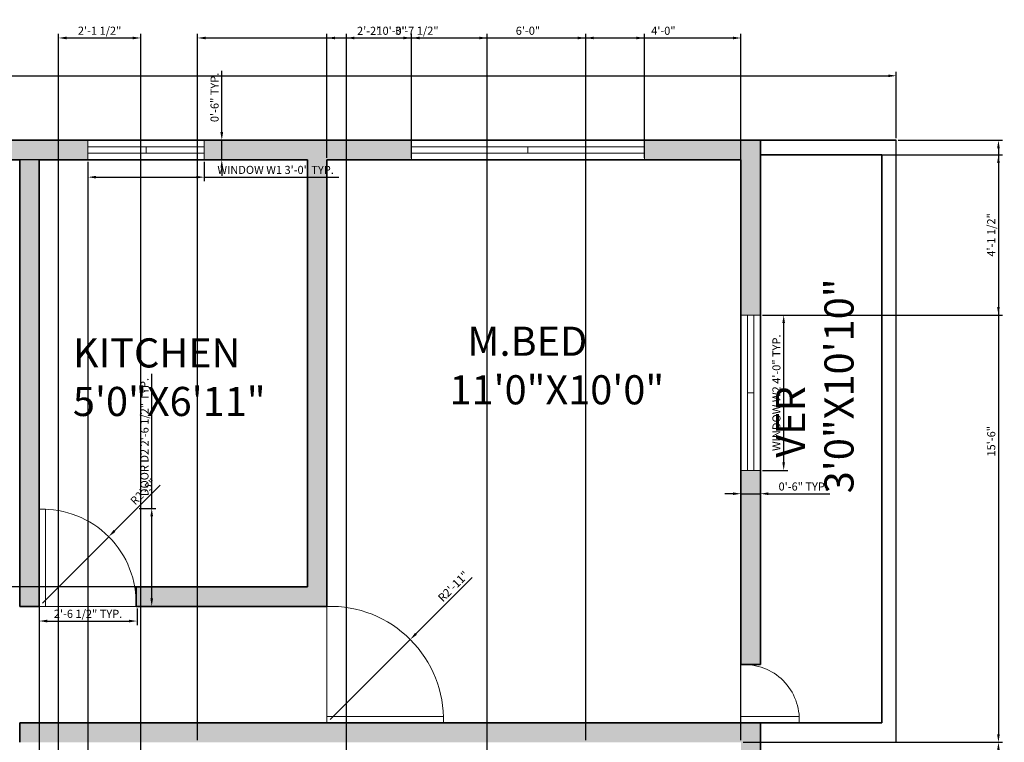
# Model space of a CAD drawing. Units: inches. Extents: x 5145 to 5807, y 9597 to 10060.
# Tile 3 of 3: x 5502 to 5807, y 9836 to 10060. Entities that reach past the tile are written whole.
import ezdxf

# ---------------------------------------------------------------- set-up
doc = ezdxf.new("R2010")
doc.units = ezdxf.units.IN
for name, color, linetype, lineweight in [('A-ANNO-DIMS', 7, 'Continuous', 18), ('A-AREA-IDEN', 7, 'Continuous', 18), ('A-GLAZ', 140, 'Continuous', 18), ('A-WALL', 7, 'Continuous', 35)]:
    doc.layers.add(name, color=color, linetype=linetype, lineweight=lineweight)
for name, color, linetype, lineweight, true_color in [('A-DOOR', 2, 'Continuous', 18, 0xf1eb1f), ('A-WALL-PATT', 159, 'Continuous', 13, 0x22346e), ('A-WALL-PRPT', 61, 'Continuous', 25, 0xedee99)]:
    doc.layers.add(name, color=color, linetype=linetype, lineweight=lineweight, true_color=true_color)
doc.styles.get("Standard").update_dxf_attribs({"font": 'arial.ttf'})
doc.dimstyles.new('ISO-25', dxfattribs={"dimtxt": 2.5, "dimasz": 2.5, "dimexe": 1.25, "dimexo": 0.625, "dimtad": 1, "dimlunit": 3, "dimtxsty": 'Standard', "dimcen": 2.5, "dimadec": 0, "dimazin": 0, "dimtfac": 1, "dimtmove": 0, "dimatfit": 3, "dimfxl": 1, "dimarcsym": 0})

# ---------------------------------------------------------------- blocks, each defined once
blk = doc.blocks.new('*D1')
at = {"layer": 'A-ANNO-DIMS', "color": 0, "lineweight": -2, "transparency": 16777216}
for p, q in [((5182.12, 10022.89), (5182.12, 10043.44)), ((5773.12, 10022.89), (5773.12, 10043.44)), ((5184.62, 10042.19), (5770.62, 10042.19))]:
    blk.add_line(p, q, dxfattribs=at)
at = {"layer": 'A-ANNO-DIMS', "color": 0, "transparency": 16777216}
for points in [[(5184.62, 10042.6), (5184.62, 10041.77), (5182.12, 10042.19)], [(5770.62, 10042.6), (5770.62, 10041.77), (5773.12, 10042.19)]]:
    blk.add_solid(points, dxfattribs=at)
at = {"layer": 'Defpoints', "color": 0, "transparency": 16777216}
for p in [(5773.12, 10042.19), (5182.12, 10022.27), (5773.12, 10022.27)]:
    blk.add_point(p, dxfattribs=at)
at = {"layer": 'A-ANNO-DIMS', "color": 0, "transparency": 16777216, "insert": (5477.62, 10047.41), "char_height": 9, "attachment_point": 5}
blk.add_mtext('49\'-3"', dxfattribs=at)
blk = doc.blocks.new('WIN-36IN')
for p, q in [((0, 6), (0, 0)), ((0, 6), (36, 6)), ((0, 4), (36, 4)), ((18, 2), (18, 4)), ((36, 0), (36, 6)), ((0, 2), (36, 2)), ((36, 0), (0, 0))]:
    blk.add_line(p, q)
blk = doc.blocks.new('WIN-48IN')
for p, q in [((6, 48), (0, 48)), ((0, 48), (0, 0)), ((2, 0), (2, 48)), ((4, 0), (4, 48)), ((6, 0), (6, 48)), ((4, 24), (2, 24)), ((0, 0), (6, 0))]:
    blk.add_line(p, q)
blk = doc.blocks.new('DOOR-SWING-18IN')
for p, q in [((0.03, 18.03), (18.03, 18.03)), ((16.03, 0.03), (16.03, 18.03)), ((16.03, 18.03), (18.03, 18.03)), ((18.03, 18.03), (18.03, 0.03)), ((18.03, 0.03), (16.03, 0.03))]:
    blk.add_line(p, q)
blk.add_arc((17.03, 17.03), 17.03, 176.6335, 273.3665)
blk = doc.blocks.new('DOOR-SWING-30IN')
for p, q in [((0, 0), (0, 30)), ((0, 30), (2, 30)), ((2, 30), (2, 0)), ((2, 0), (0, 0)), ((0, 0), (30, 0))]:
    blk.add_line(p, q)
blk.add_arc((1, 1), 29.02, 358.0251, 91.9749)
blk = doc.blocks.new('*D9')
at = {"layer": 'A-ANNO-DIMS', "color": 0, "lineweight": -2, "transparency": 16777216}
for p, q in [((5523.2, 10015.64), (5523.2, 10009.62)), ((5559.2, 10015.64), (5559.2, 10009.62)), ((5525.7, 10010.87), (5556.7, 10010.87)), ((5559.2, 10010.87), (5600.79, 10010.87))]:
    blk.add_line(p, q, dxfattribs=at)
at = {"layer": 'A-ANNO-DIMS', "color": 0, "transparency": 16777216}
for points in [[(5525.7, 10011.28), (5525.7, 10010.45), (5523.2, 10010.87)], [(5556.7, 10011.28), (5556.7, 10010.45), (5559.2, 10010.87)]]:
    blk.add_solid(points, dxfattribs=at)
at = {"layer": 'Defpoints', "color": 0, "transparency": 16777216}
for p in [(5523.2, 10016.27), (5559.2, 10016.27), (5559.2, 10010.87)]:
    blk.add_point(p, dxfattribs=at)
at = {"layer": 'A-ANNO-DIMS', "color": 0, "transparency": 16777216, "insert": (5581.24, 10012.79), "char_height": 2.5, "attachment_point": 5}
blk.add_mtext('WINDOW W1 3\'-0" TYP.', dxfattribs=at)
blk = doc.blocks.new('*D10')
at = {"layer": 'A-ANNO-DIMS', "color": 0, "lineweight": -2, "transparency": 16777216}
for p, q in [((5564.6, 10024.77), (5564.6, 10043.76)), ((5559.82, 10022.27), (5565.85, 10022.27)), ((5564.6, 10016.27), (5564.6, 10022.27)), ((5559.82, 10016.27), (5565.85, 10016.27)), ((5564.6, 10013.77), (5564.6, 10011.27))]:
    blk.add_line(p, q, dxfattribs=at)
at = {"layer": 'A-ANNO-DIMS', "color": 0, "transparency": 16777216}
for points in [[(5564.18, 10024.77), (5565.01, 10024.77), (5564.6, 10022.27)], [(5564.18, 10013.77), (5565.01, 10013.77), (5564.6, 10016.27)]]:
    blk.add_solid(points, dxfattribs=at)
at = {"layer": 'Defpoints', "color": 0, "transparency": 16777216}
for p in [(5559.2, 10022.27), (5564.6, 10022.27), (5559.2, 10016.27)]:
    blk.add_point(p, dxfattribs=at)
at = {"layer": 'A-ANNO-DIMS', "color": 0, "transparency": 16777216, "insert": (5562.69, 10035.51), "char_height": 2.5, "attachment_point": 5, "rotation": 90}
blk.add_mtext('0\'-6" TYP.', dxfattribs=at)
blk = doc.blocks.new('*D11')
at = {"layer": 'A-ANNO-DIMS', "color": 0, "lineweight": -2, "transparency": 16777216}
for p, q in [((5731.74, 9968.27), (5739.57, 9968.27)), ((5738.32, 9922.77), (5738.32, 9965.77)), ((5731.74, 9920.27), (5739.57, 9920.27))]:
    blk.add_line(p, q, dxfattribs=at)
at = {"layer": 'A-ANNO-DIMS', "color": 0, "transparency": 16777216}
for points in [[(5737.9, 9965.77), (5738.73, 9965.77), (5738.32, 9968.27)], [(5737.9, 9922.77), (5738.73, 9922.77), (5738.32, 9920.27)]]:
    blk.add_solid(points, dxfattribs=at)
at = {"layer": 'Defpoints', "color": 0, "transparency": 16777216}
for p in [(5731.12, 9968.27), (5738.32, 9968.27), (5731.12, 9920.27)]:
    blk.add_point(p, dxfattribs=at)
at = {"layer": 'A-ANNO-DIMS', "color": 0, "transparency": 16777216, "insert": (5736.4, 9944.27), "char_height": 2.5, "attachment_point": 5, "rotation": 90}
blk.add_mtext('WINDOW W2 4\'-0" TYP.', dxfattribs=at)
blk = doc.blocks.new('*D12')
at = {"layer": 'A-ANNO-DIMS', "color": 0, "lineweight": -2, "transparency": 16777216}
for p, q in [((5725.12, 9919.64), (5725.12, 9911.82)), ((5731.12, 9919.64), (5731.12, 9911.82)), ((5722.62, 9913.07), (5720.12, 9913.07)), ((5725.12, 9913.07), (5731.12, 9913.07)), ((5733.62, 9913.07), (5752.61, 9913.07))]:
    blk.add_line(p, q, dxfattribs=at)
at = {"layer": 'A-ANNO-DIMS', "color": 0, "transparency": 16777216}
for points in [[(5722.62, 9913.48), (5722.62, 9912.65), (5725.12, 9913.07)], [(5733.62, 9913.48), (5733.62, 9912.65), (5731.12, 9913.07)]]:
    blk.add_solid(points, dxfattribs=at)
at = {"layer": 'Defpoints', "color": 0, "transparency": 16777216}
for p in [(5725.12, 9920.27), (5731.12, 9920.27), (5731.12, 9913.07)]:
    blk.add_point(p, dxfattribs=at)
at = {"layer": 'A-ANNO-DIMS', "color": 0, "transparency": 16777216, "insert": (5744.36, 9914.97), "char_height": 2.5, "attachment_point": 5}
blk.add_mtext('0\'-6" TYP.', dxfattribs=at)
blk = doc.blocks.new('*D17')
at = {"layer": 'A-ANNO-DIMS', "color": 0, "lineweight": -2, "transparency": 16777216}
for p, q in [((5542.94, 9908.54), (5542.94, 9950.12)), ((5539.02, 9908.54), (5544.19, 9908.54)), ((5542.94, 9880.77), (5542.94, 9906.04)), ((5539.02, 9878.27), (5544.19, 9878.27))]:
    blk.add_line(p, q, dxfattribs=at)
at = {"layer": 'A-ANNO-DIMS', "color": 0, "transparency": 16777216}
for points in [[(5542.52, 9906.04), (5543.35, 9906.04), (5542.94, 9908.54)], [(5542.52, 9880.77), (5543.35, 9880.77), (5542.94, 9878.27)]]:
    blk.add_solid(points, dxfattribs=at)
at = {"layer": 'Defpoints', "color": 0, "transparency": 16777216}
for p in [(5538.39, 9908.54), (5542.94, 9908.54), (5538.39, 9878.27)]:
    blk.add_point(p, dxfattribs=at)
at = {"layer": 'A-ANNO-DIMS', "color": 0, "transparency": 16777216, "insert": (5541.02, 9930.58), "char_height": 2.5, "attachment_point": 5, "rotation": 90}
blk.add_mtext('DOOR D2 2\'-6 1/2" TYP.', dxfattribs=at)
blk = doc.blocks.new('*D18')
at = {"layer": 'A-ANNO-DIMS', "color": 0, "lineweight": -2, "transparency": 16777216}
for p, q in [((5508.12, 9877.64), (5508.12, 9872.48)), ((5538.39, 9877.64), (5538.39, 9872.48)), ((5510.62, 9873.73), (5535.89, 9873.73))]:
    blk.add_line(p, q, dxfattribs=at)
at = {"layer": 'A-ANNO-DIMS', "color": 0, "transparency": 16777216}
for points in [[(5510.62, 9874.14), (5510.62, 9873.31), (5508.12, 9873.73)], [(5535.89, 9874.14), (5535.89, 9873.31), (5538.39, 9873.73)]]:
    blk.add_solid(points, dxfattribs=at)
at = {"layer": 'Defpoints', "color": 0, "transparency": 16777216}
for p in [(5508.12, 9878.27), (5538.39, 9878.27), (5538.39, 9873.73)]:
    blk.add_point(p, dxfattribs=at)
at = {"layer": 'A-ANNO-DIMS', "color": 0, "transparency": 16777216, "insert": (5523.25, 9875.64), "char_height": 2.5, "attachment_point": 5}
blk.add_mtext('2\'-6 1/2" TYP.', dxfattribs=at)
blk = doc.blocks.new('*D27')
at = {"layer": 'A-ANNO-DIMS', "color": 0, "lineweight": -2, "transparency": 16777216}
for p, q in [((5773.74, 10022.27), (5805.97, 10022.27)), ((5804.72, 10019.77), (5804.72, 9838.77)), ((5773.74, 9836.27), (5805.97, 9836.27))]:
    blk.add_line(p, q, dxfattribs=at)
at = {"layer": 'A-ANNO-DIMS', "color": 0, "transparency": 16777216}
for points in [[(5804.3, 10019.77), (5805.13, 10019.77), (5804.72, 10022.27)], [(5804.3, 9838.77), (5805.13, 9838.77), (5804.72, 9836.27)]]:
    blk.add_solid(points, dxfattribs=at)
at = {"layer": 'Defpoints', "color": 0, "transparency": 16777216}
for p in [(5773.12, 10022.27), (5773.12, 9836.27), (5804.72, 9836.27)]:
    blk.add_point(p, dxfattribs=at)
at = {"layer": 'A-ANNO-DIMS', "color": 0, "transparency": 16777216, "insert": (5802.81, 9929.27), "char_height": 2.5, "attachment_point": 5, "rotation": 90}
blk.add_mtext('15\'-6"', dxfattribs=at)
blk = doc.blocks.new('*D29')
at = {"layer": 'A-ANNO-DIMS', "color": 0, "lineweight": -2, "transparency": 16777216}
for p, q in [((5590.49, 10016.27), (5149.27, 10016.27)), ((5150.52, 10013.77), (5150.52, 9886.77)), ((5590.49, 9884.27), (5149.27, 9884.27))]:
    blk.add_line(p, q, dxfattribs=at)
at = {"layer": 'A-ANNO-DIMS', "color": 0, "transparency": 16777216}
for points in [[(5150.1, 10013.77), (5150.93, 10013.77), (5150.52, 10016.27)], [(5150.1, 9886.77), (5150.93, 9886.77), (5150.52, 9884.27)]]:
    blk.add_solid(points, dxfattribs=at)
at = {"layer": 'Defpoints', "color": 0, "transparency": 16777216}
for p in [(5591.12, 10016.27), (5150.52, 9884.27), (5591.12, 9884.27)]:
    blk.add_point(p, dxfattribs=at)
at = {"layer": 'A-ANNO-DIMS', "color": 0, "transparency": 16777216, "insert": (5148.61, 9950.27), "char_height": 2.5, "attachment_point": 5, "rotation": 90}
blk.add_mtext('11\'-0"', dxfattribs=at)
blk = doc.blocks.new('*D31')
at = {"layer": 'A-ANNO-DIMS', "color": 0, "lineweight": -2, "transparency": 16777216}
for p, q in [((5557.12, 9836.89), (5557.12, 10055.12)), ((5677.12, 9836.89), (5677.12, 10055.12)), ((5559.62, 10053.87), (5674.62, 10053.87))]:
    blk.add_line(p, q, dxfattribs=at)
at = {"layer": 'A-ANNO-DIMS', "color": 0, "transparency": 16777216}
for points in [[(5559.62, 10054.28), (5559.62, 10053.45), (5557.12, 10053.87)], [(5674.62, 10054.28), (5674.62, 10053.45), (5677.12, 10053.87)]]:
    blk.add_solid(points, dxfattribs=at)
at = {"layer": 'Defpoints', "color": 0, "transparency": 16777216}
for p in [(5677.12, 10053.87), (5557.12, 9836.27), (5677.12, 9836.27)]:
    blk.add_point(p, dxfattribs=at)
at = {"layer": 'A-ANNO-DIMS', "color": 0, "transparency": 16777216, "insert": (5617.12, 10055.77), "char_height": 2.5, "attachment_point": 5}
blk.add_mtext('10\'-0"', dxfattribs=at)
blk = doc.blocks.new('*D32')
at = {"layer": 'A-ANNO-DIMS', "color": 0, "lineweight": -2, "transparency": 16777216}
for p, q in [((5677.12, 9836.89), (5677.12, 10055.12)), ((5725.12, 9836.89), (5725.12, 10055.12)), ((5679.62, 10053.87), (5722.62, 10053.87))]:
    blk.add_line(p, q, dxfattribs=at)
at = {"layer": 'A-ANNO-DIMS', "color": 0, "transparency": 16777216}
for points in [[(5679.62, 10054.28), (5679.62, 10053.45), (5677.12, 10053.87)], [(5722.62, 10054.28), (5722.62, 10053.45), (5725.12, 10053.87)]]:
    blk.add_solid(points, dxfattribs=at)
at = {"layer": 'Defpoints', "color": 0, "transparency": 16777216}
for p in [(5725.12, 10053.87), (5677.12, 9836.27), (5725.12, 9836.27)]:
    blk.add_point(p, dxfattribs=at)
at = {"layer": 'A-ANNO-DIMS', "color": 0, "transparency": 16777216, "insert": (5701.12, 10055.77), "char_height": 2.5, "attachment_point": 5}
blk.add_mtext('4\'-0"', dxfattribs=at)
blk = doc.blocks.new('*D37')
at = {"layer": 'A-ANNO-DIMS', "color": 0, "lineweight": -2, "transparency": 16777216}
for p, q in [((5508.12, 10015.64), (5508.12, 9597.42)), ((5523.2, 10015.64), (5523.2, 9597.42)), ((5510.62, 9598.67), (5520.7, 9598.67))]:
    blk.add_line(p, q, dxfattribs=at)
at = {"layer": 'A-ANNO-DIMS', "color": 0, "transparency": 16777216}
for points in [[(5510.62, 9599.08), (5510.62, 9598.25), (5508.12, 9598.67)], [(5520.7, 9599.08), (5520.7, 9598.25), (5523.2, 9598.67)]]:
    blk.add_solid(points, dxfattribs=at)
at = {"layer": 'Defpoints', "color": 0, "transparency": 16777216}
for p in [(5508.12, 10016.27), (5523.2, 10016.27), (5523.2, 9598.67)]:
    blk.add_point(p, dxfattribs=at)
at = {"layer": 'A-ANNO-DIMS', "color": 0, "transparency": 16777216, "insert": (5515.66, 9600.57), "char_height": 2.5, "attachment_point": 5}
blk.add_mtext('1\'-3"', dxfattribs=at)
blk = doc.blocks.new('*D38')
at = {"layer": 'A-ANNO-DIMS', "color": 0, "lineweight": -2, "transparency": 16777216}
for p, q in [((5597.12, 10016.89), (5597.12, 10055.12)), ((5623.25, 10016.89), (5623.25, 10055.12)), ((5599.62, 10053.87), (5620.75, 10053.87))]:
    blk.add_line(p, q, dxfattribs=at)
at = {"layer": 'A-ANNO-DIMS', "color": 0, "transparency": 16777216}
for points in [[(5599.62, 10054.28), (5599.62, 10053.45), (5597.12, 10053.87)], [(5620.75, 10054.28), (5620.75, 10053.45), (5623.25, 10053.87)]]:
    blk.add_solid(points, dxfattribs=at)
at = {"layer": 'Defpoints', "color": 0, "transparency": 16777216}
for p in [(5623.25, 10053.87), (5597.12, 10016.27), (5623.25, 10016.27)]:
    blk.add_point(p, dxfattribs=at)
at = {"layer": 'A-ANNO-DIMS', "color": 0, "transparency": 16777216, "insert": (5610.18, 10055.75), "char_height": 2.5, "attachment_point": 5}
blk.add_mtext('2\'-2"', dxfattribs=at)
blk = doc.blocks.new('*D39')
at = {"layer": 'A-ANNO-DIMS', "color": 0, "lineweight": -2, "transparency": 16777216}
for p, q in [((5623.25, 10016.89), (5623.25, 10055.12)), ((5695.25, 10016.89), (5695.25, 10055.12)), ((5625.75, 10053.87), (5692.75, 10053.87))]:
    blk.add_line(p, q, dxfattribs=at)
at = {"layer": 'A-ANNO-DIMS', "color": 0, "transparency": 16777216}
for points in [[(5625.75, 10054.28), (5625.75, 10053.45), (5623.25, 10053.87)], [(5692.75, 10054.28), (5692.75, 10053.45), (5695.25, 10053.87)]]:
    blk.add_solid(points, dxfattribs=at)
at = {"layer": 'Defpoints', "color": 0, "transparency": 16777216}
for p in [(5695.25, 10053.87), (5623.25, 10016.27), (5695.25, 10016.27)]:
    blk.add_point(p, dxfattribs=at)
at = {"layer": 'A-ANNO-DIMS', "color": 0, "transparency": 16777216, "insert": (5659.25, 10055.77), "char_height": 2.5, "attachment_point": 5}
blk.add_mtext('6\'-0"', dxfattribs=at)
blk = doc.blocks.new('*D43')
at = {"layer": 'A-ANNO-DIMS', "color": 0, "lineweight": -2, "transparency": 16777216}
for p, q in [((5514.12, 9636.89), (5514.12, 10055.12)), ((5539.54, 9636.89), (5539.54, 10055.12)), ((5516.62, 10053.87), (5537.04, 10053.87))]:
    blk.add_line(p, q, dxfattribs=at)
at = {"layer": 'A-ANNO-DIMS', "color": 0, "transparency": 16777216}
for points in [[(5516.62, 10054.28), (5516.62, 10053.45), (5514.12, 10053.87)], [(5537.04, 10054.28), (5537.04, 10053.45), (5539.54, 10053.87)]]:
    blk.add_solid(points, dxfattribs=at)
at = {"layer": 'Defpoints', "color": 0, "transparency": 16777216}
for p in [(5539.54, 10053.87), (5514.12, 9636.27), (5539.54, 9636.27)]:
    blk.add_point(p, dxfattribs=at)
at = {"layer": 'A-ANNO-DIMS', "color": 0, "transparency": 16777216, "insert": (5526.83, 10055.79), "char_height": 2.5, "attachment_point": 5}
blk.add_mtext('2\'-1 1/2"', dxfattribs=at)
blk = doc.blocks.new('*D44')
at = {"layer": 'A-ANNO-DIMS', "color": 0, "lineweight": -2, "transparency": 16777216}
for p, q in [((5603.12, 9636.89), (5603.12, 10055.12)), ((5646.69, 9636.89), (5646.69, 10055.12)), ((5605.62, 10053.87), (5644.19, 10053.87))]:
    blk.add_line(p, q, dxfattribs=at)
at = {"layer": 'A-ANNO-DIMS', "color": 0, "transparency": 16777216}
for points in [[(5605.62, 10054.28), (5605.62, 10053.45), (5603.12, 10053.87)], [(5644.19, 10054.28), (5644.19, 10053.45), (5646.69, 10053.87)]]:
    blk.add_solid(points, dxfattribs=at)
at = {"layer": 'Defpoints', "color": 0, "transparency": 16777216}
for p in [(5646.69, 10053.87), (5603.12, 9636.27), (5646.69, 9636.27)]:
    blk.add_point(p, dxfattribs=at)
at = {"layer": 'A-ANNO-DIMS', "color": 0, "transparency": 16777216, "insert": (5624.91, 10055.79), "char_height": 2.5, "attachment_point": 5}
blk.add_mtext('3\'-7 1/2"', dxfattribs=at)
blk = doc.blocks.new('*D47')
at = {"layer": 'A-ANNO-DIMS', "color": 0, "lineweight": -2, "transparency": 16777216}
for p, q in [((5731.74, 10017.77), (5805.97, 10017.77)), ((5804.72, 10015.27), (5804.72, 9970.77)), ((5731.74, 9968.27), (5805.97, 9968.27))]:
    blk.add_line(p, q, dxfattribs=at)
at = {"layer": 'A-ANNO-DIMS', "color": 0, "transparency": 16777216}
for points in [[(5804.3, 10015.27), (5805.13, 10015.27), (5804.72, 10017.77)], [(5804.3, 9970.77), (5805.13, 9970.77), (5804.72, 9968.27)]]:
    blk.add_solid(points, dxfattribs=at)
at = {"layer": 'Defpoints', "color": 0, "transparency": 16777216}
for p in [(5731.12, 10017.77), (5731.12, 9968.27), (5804.72, 9968.27)]:
    blk.add_point(p, dxfattribs=at)
at = {"layer": 'A-ANNO-DIMS', "color": 0, "transparency": 16777216, "insert": (5802.8, 9993.02), "char_height": 2.5, "attachment_point": 5, "rotation": 90}
blk.add_mtext('4\'-1 1/2"', dxfattribs=at)
blk = doc.blocks.new('*D48')
at = {"layer": 'A-ANNO-DIMS', "color": 0, "lineweight": -2, "transparency": 16777216}
for p, q in [((5725.74, 9836.27), (5805.97, 9836.27)), ((5804.72, 9833.77), (5804.72, 9816.96)), ((5725.74, 9814.46), (5805.97, 9814.46))]:
    blk.add_line(p, q, dxfattribs=at)
at = {"layer": 'A-ANNO-DIMS', "color": 0, "transparency": 16777216}
for points in [[(5804.3, 9833.77), (5805.13, 9833.77), (5804.72, 9836.27)], [(5804.3, 9816.96), (5805.13, 9816.96), (5804.72, 9814.46)]]:
    blk.add_solid(points, dxfattribs=at)
at = {"layer": 'Defpoints', "color": 0, "transparency": 16777216}
for p in [(5725.12, 9836.27), (5725.12, 9814.46), (5804.72, 9814.46)]:
    blk.add_point(p, dxfattribs=at)
at = {"layer": 'A-ANNO-DIMS', "color": 0, "transparency": 16777216, "insert": (5802.81, 9825.36), "char_height": 2.5, "attachment_point": 5, "rotation": 90}
blk.add_mtext('1\'-10"', dxfattribs=at)
blk = doc.blocks.new('*D53')
at = {"layer": 'A-ANNO-DIMS', "color": 0, "lineweight": -2, "transparency": 16777216}
for p, q in [((5642.05, 9887.21), (5624.64, 9869.79)), ((5598.12, 9843.27), (5622.88, 9868.03))]:
    blk.add_line(p, q, dxfattribs=at)
at = {"layer": 'A-ANNO-DIMS', "color": 0, "transparency": 16777216}
blk.add_solid([(5624.35, 9870.09), (5624.94, 9869.5), (5622.88, 9868.03)], dxfattribs=at)
at = {"layer": 'Defpoints', "color": 0, "transparency": 16777216}
for p in [(5622.88, 9868.03), (5598.12, 9843.27)]:
    blk.add_point(p, dxfattribs=at)
at = {"layer": 'A-ANNO-DIMS', "color": 0, "transparency": 16777216, "insert": (5636.4, 9884.21), "char_height": 2.5, "attachment_point": 5, "rotation": 45}
blk.add_mtext('R2\'-11"', dxfattribs=at)
blk = doc.blocks.new('*D54')
at = {"layer": 'A-ANNO-DIMS', "color": 0, "lineweight": -2, "transparency": 16777216}
for p, q in [((5545.58, 9915.73), (5531.4, 9901.55)), ((5509.12, 9879.27), (5529.63, 9899.79))]:
    blk.add_line(p, q, dxfattribs=at)
at = {"layer": 'A-ANNO-DIMS', "color": 0, "transparency": 16777216}
blk.add_solid([(5531.11, 9901.85), (5531.7, 9901.26), (5529.63, 9899.79)], dxfattribs=at)
at = {"layer": 'Defpoints', "color": 0, "transparency": 16777216}
for p in [(5529.63, 9899.79), (5509.12, 9879.27)]:
    blk.add_point(p, dxfattribs=at)
at = {"layer": 'A-ANNO-DIMS', "color": 0, "transparency": 16777216, "insert": (5540.6, 9913.44), "char_height": 2.5, "attachment_point": 5, "rotation": 45}
blk.add_mtext('R2\'-5"', dxfattribs=at)

msp = doc.modelspace()

# ---------------------------------------------------------------- hatches: boundary and pattern name
at = {"layer": 'A-WALL-PATT'}
h = msp.add_hatch(color=256, dxfattribs=at)
h.dxf.hatch_style = 1
h.paths.add_polyline_path([(5244.116, 10016.267), (5266.307, 10016.267), (5266.307, 10022.267), (5238.116, 10022.267), (5238.116, 10017.767), (5238.116, 9962.267), (5329.116, 9962.267), (5329.116, 9968.267), (5311.116, 9968.267), (5244.116, 9968.267)])
h.paths.add_polyline_path([(5372.995, 10022.267), (5290.307, 10022.267), (5290.307, 10016.267), (5323.116, 10016.267), (5323.116, 9986.267), (5327.116, 9986.267, -0.0293864), (5329.116, 9986.267), (5329.116, 10016.267), (5372.995, 10016.267)])
h.paths.add_polyline_path([(5523.196, 10022.267), (5432.995, 10022.267), (5432.995, 10016.267), (5502.116, 10016.267), (5502.116, 9878.267), (5508.116, 9878.267), (5508.116, 9908.267), (5508.116, 10016.267), (5523.196, 10016.267)])
h.paths.add_polyline_path([(5623.247, 10022.267), (5559.196, 10022.267), (5559.196, 10016.267), (5591.116, 10016.267), (5591.116, 9884.267), (5538.116, 9884.267), (5538.116, 9880.267, -0.0172363), (5538.116, 9878.267), (5597.116, 9878.267), (5597.116, 10016.267), (5623.247, 10016.267)])
h.paths.add_polyline_path([(5731.116, 10022.267), (5695.247, 10022.267), (5695.247, 10016.267), (5725.116, 10016.267), (5725.116, 9968.267), (5731.116, 9968.267)])
h.paths.add_polyline_path([(5731.116, 9920.267), (5725.116, 9920.267), (5725.116, 9860.267, -0.0293864), (5727.116, 9860.267), (5731.116, 9860.267)])
h.paths.add_polyline_path([(5731.116, 9842.267), (5725.116, 9842.267), (5502.116, 9842.267), (5502.116, 9836.267), (5725.116, 9836.267), (5725.116, 9814.459), (5731.116, 9814.459)])
h.paths.add_polyline_path([(5731.116, 9778.459), (5725.116, 9778.459), (5725.116, 9752.267), (5502.116, 9752.267), (5502.116, 9746.267), (5731.116, 9746.267)])
h.paths.add_polyline_path([(5514.116, 9717.93), (5508.116, 9717.93), (5508.116, 9704.267), (5508.116, 9636.267), (5460.439, 9636.267), (5460.439, 9630.267), (5539.543, 9630.267), (5539.543, 9636.267), (5514.116, 9636.267), (5514.116, 9704.267)])
h.paths.add_polyline_path([(5603.116, 9717.93), (5544.116, 9717.93, -0.0172363), (5544.116, 9715.93), (5544.116, 9711.93), (5597.116, 9711.93), (5597.116, 9636.267), (5575.543, 9636.267), (5575.543, 9630.267), (5646.695, 9630.267), (5646.695, 9636.267), (5603.116, 9636.267), (5603.116, 9704.267)])
h.paths.add_polyline_path([(5731.116, 9649.987), (5725.116, 9649.987), (5725.116, 9636.267), (5694.695, 9636.267), (5694.695, 9630.267), (5731.116, 9630.267)])
h.paths.add_polyline_path([(5731.116, 9728.267), (5725.116, 9728.267), (5725.116, 9685.987), (5731.116, 9685.987)])
h.paths.add_polyline_path([(5400.439, 9636.267), (5329.116, 9636.267), (5329.116, 9662.267, -0.0217289), (5327.116, 9662.267), (5323.116, 9662.267), (5323.116, 9636.267), (5283.616, 9636.267), (5283.616, 9630.267), (5329.116, 9630.267), (5400.439, 9630.267)])
h.paths.add_polyline_path([(5263.165, 9636.267), (5244.116, 9636.267), (5244.116, 9686.267), (5329.116, 9686.267), (5329.116, 9692.267), (5287.116, 9692.267), (5238.116, 9692.267), (5238.116, 9674.267), (5238.116, 9630.267), (5263.165, 9630.267)])
h.paths.add_polyline_path([(5220.116, 9690.267, -0.0293864), (5220.116, 9692.267), (5188.116, 9692.267), (5188.116, 9734.135), (5182.116, 9734.135), (5182.116, 9686.267), (5220.116, 9686.267)])
h.paths.add_polyline_path([(5329.116, 9794.267), (5469.593, 9794.267), (5469.593, 9800.267), (5427.593, 9800.267), (5329.116, 9800.267), (5329.116, 9830.267), (5329.116, 9920.267, -0.0121933), (5327.116, 9920.267), (5323.116, 9920.267), (5323.116, 9830.267), (5188.116, 9830.267), (5188.116, 9865.614), (5182.116, 9865.614), (5182.116, 9794.135), (5188.116, 9794.135), (5188.116, 9824.267), (5323.116, 9824.267), (5323.116, 9734.267), (5327.116, 9734.267, -0.0121933), (5329.116, 9734.267)])

# ---------------------------------------------------------------- linework, layer by layer
at = {"layer": 'A-DOOR'}
for p, q in [((5597.116, 9842.267), (5597.116, 9878.267)), ((5633.116, 9844.267), (5597.116, 9844.267)), ((5597.116, 9844.267), (5597.116, 9842.267)), ((5597.116, 9842.267), (5633.116, 9842.267)), ((5633.116, 9842.267), (5633.116, 9844.267))]:
    msp.add_line(p, q, dxfattribs=at)
msp.add_arc((5598.116, 9843.267), 35.014, 358.36342, 91.63658, dxfattribs=at)
at = {"layer": 'A-GLAZ'}
for p, q in [((5523.196, 10022.267), (5523.196, 10016.267)), ((5523.196, 10022.267), (5559.196, 10022.267)), ((5523.196, 10022.267), (5559.196, 10022.267)), ((5523.196, 10022.267), (5559.196, 10022.267)), ((5559.196, 10022.267), (5559.196, 10016.267)), ((5623.247, 10022.267), (5623.247, 10016.267)), ((5695.247, 10022.267), (5623.247, 10022.267)), ((5623.247, 10022.267), (5662.116, 10022.267)), ((5623.247, 10022.267), (5623.247, 10016.267)), ((5695.247, 10016.267), (5695.247, 10022.267)), ((5695.247, 10016.267), (5695.247, 10022.267)), ((5695.247, 10020.267), (5623.247, 10020.267)), ((5695.247, 10018.267), (5623.247, 10018.267)), ((5659.247, 10018.267), (5659.247, 10020.267)), ((5523.196, 10016.267), (5559.196, 10016.267)), ((5623.247, 10016.267), (5695.247, 10016.267)), ((5623.247, 10016.267), (5695.247, 10016.267)), ((5731.116, 9968.267), (5725.116, 9968.267)), ((5731.116, 9920.267), (5731.116, 9968.267)), ((5731.116, 9920.267), (5725.116, 9920.267))]:
    msp.add_line(p, q, dxfattribs=at)
at = {"layer": 'A-WALL'}
for p, q in [((5182.116, 10022.267), (5662.116, 10022.267)), ((5773.116, 10022.267), (5662.116, 10022.267)), ((5731.116, 9860.267), (5731.116, 10022.267)), ((5329.116, 10016.267), (5502.116, 10016.267)), ((5502.116, 9878.267), (5502.116, 10016.267)), ((5508.116, 10016.267), (5591.116, 10016.267)), ((5508.116, 9878.267), (5508.116, 10016.267)), ((5591.116, 9884.267), (5591.116, 10016.267)), ((5597.116, 10016.267), (5725.116, 10016.267)), ((5597.116, 9878.267), (5597.116, 10016.267)), ((5725.116, 9860.267), (5725.116, 10016.267)), ((5538.116, 9884.267), (5591.116, 9884.267)), ((5538.116, 9878.267), (5538.116, 9884.267)), ((5538.116, 9884.267), (5591.116, 9884.267)), ((5508.116, 9878.267), (5502.116, 9878.267)), ((5538.116, 9878.267), (5597.116, 9878.267)), ((5725.116, 9860.267), (5731.116, 9860.267)), ((5502.116, 9842.267), (5731.116, 9842.267)), ((5502.116, 9842.267), (5502.116, 9836.267)), ((5725.116, 9842.267), (5767.116, 9842.267)), ((5731.116, 9746.267), (5731.116, 9842.267))]:
    msp.add_line(p, q, dxfattribs=at)
at = {"layer": 'A-WALL-PRPT'}
for p, q in [((5773.116, 10022.267), (5731.116, 10022.267)), ((5773.116, 10016.267), (5773.116, 10022.267)), ((5773.116, 9836.267), (5773.116, 10022.267)), ((5768.616, 10017.767), (5731.116, 10017.767)), ((5731.116, 10017.767), (5768.616, 10017.767)), ((5768.616, 9882.767), (5768.616, 10017.767)), ((5768.616, 10017.767), (5768.616, 9842.267)), ((5773.116, 9878.267), (5773.116, 10016.267)), ((5768.616, 9842.267), (5768.616, 9882.767)), ((5773.116, 9836.267), (5773.116, 9878.267)), ((5731.116, 9842.267), (5768.616, 9842.267)), ((5768.616, 9842.267), (5731.116, 9842.267))]:
    msp.add_line(p, q, dxfattribs=at)

# ---------------------------------------------------------------- block references
at = {"layer": 'A-DOOR'}
msp.add_blockref('DOOR-SWING-30IN', (5508.116, 9878.267), dxfattribs=at)
at = {"layer": 'A-DOOR', "extrusion": (0, 0, -1), "zscale": -1, "rotation": 270.0000000000189}
msp.add_blockref('DOOR-SWING-18IN', (-5743.146, 9860.297), dxfattribs=at)
at = {"layer": 'A-GLAZ'}
for name, p in [('WIN-36IN', (5523.196, 10016.267)), ('WIN-48IN', (5725.116, 9920.267))]:
    msp.add_blockref(name, p, dxfattribs=at)

# ---------------------------------------------------------------- texts
at = {"layer": 'A-AREA-IDEN', "insert": (5735.913, 9913.196), "char_height": 9, "attachment_point": 1, "rotation": 90}
msp.add_mtext_dynamic_manual_height_columns('    VER\\P3\'0"X10\'10"', width=68.70978, gutter_width=12.5, heights=[37.922], dxfattribs=at)
at = {"layer": 'A-AREA-IDEN', "char_height": 9, "attachment_point": 1}
for s, width, heights, insert in [('  M.BED\\P11\'0"X10\'0"', 51.95741, [0], (5634.986, 9964.677)), (' KITCHEN\\P 5\'0"X6\'11"', 76.31305, [51.205], (5515.818, 9961.073))]:
    msp.add_mtext_dynamic_manual_height_columns(s, width=width, gutter_width=12.5, heights=heights, dxfattribs=dict(at, insert=insert))

# ---------------------------------------------------------------- dimensions: what is measured, and where the dimension line sits
at = {"layer": 'A-ANNO-DIMS'}
for base, p1, p2, picture, middle in [((5539.543, 10053.867), (5514.116, 9636.267), (5539.543, 9636.267), '*D43', (5526.83, 10055.785)), ((5646.695, 10053.867), (5603.116, 9636.267), (5646.695, 9636.267), '*D44', (5624.906, 10055.786)), ((5677.116, 10053.867), (5557.116, 9836.267), (5677.116, 9836.267), '*D31', (5617.116, 10055.769)), ((5623.247, 10053.867), (5597.116, 10016.267), (5623.247, 10016.267), '*D38', (5610.182, 10055.748)), ((5695.247, 10053.867), (5623.247, 10016.267), (5695.247, 10016.267), '*D39', (5659.247, 10055.769)), ((5725.116, 10053.867), (5677.116, 9836.267), (5725.116, 9836.267), '*D32', (5701.116, 10055.769)), ((5523.196, 9598.667), (5508.116, 10016.267), (5523.196, 10016.267), '*D37', (5515.656, 9600.57))]:
    dim = msp.add_linear_dim(base=base, p1=p1, p2=p2, dimstyle='ISO-25', override={"dimdec": 1, "dimlfac": 1, "dimrnd": 0, "dimzin": 1, "dimdsep": 46, "dimlunit": 4, "dimfrac": 2}, dxfattribs=at)
    dim.commit()
    dim.dimension.update_dxf_attribs({"geometry": picture, "text_midpoint": middle})
dim = msp.add_linear_dim(base=(5773.116, 10042.186), p1=(5182.116, 10022.267), p2=(5773.116, 10022.267), dimstyle='ISO-25', override={"dimtxt": 9, "dimclrd": 0, "dimclre": 0, "dimclrt": 0}, dxfattribs=at)
dim.commit()
dim.dimension.update_dxf_attribs({"geometry": '*D1', "text_midpoint": (5477.616, 10042.186), "dimtype": 160})
for base, p1, p2, text, picture, middle in [((5564.596, 10022.267), (5559.196, 10016.267), (5559.196, 10022.267), '<> TYP.', '*D10', (5562.695, 10035.512)), ((5738.316, 9968.267), (5731.116, 9920.267), (5731.116, 9968.267), 'WINDOW W2 <> TYP.', '*D11', (5736.398, 9944.267)), ((5542.935, 9908.545), (5538.394, 9878.267), (5538.394, 9908.545), 'DOOR D2 <> TYP.', '*D17', (5541.017, 9930.581))]:
    dim = msp.add_linear_dim(base=base, p1=p1, p2=p2, angle=90, text=text, dimstyle='ISO-25', override={"dimdec": 1, "dimlfac": 1, "dimrnd": 0, "dimzin": 1, "dimdsep": 46, "dimlunit": 4, "dimfrac": 2}, dxfattribs=at)
    dim.commit()
    dim.dimension.update_dxf_attribs({"geometry": picture, "text_midpoint": middle})
for base, p1, p2, picture, middle in [((5804.716, 9836.267), (5773.116, 10022.267), (5773.116, 9836.267), '*D27', (5802.815, 9929.267)), ((5150.516, 9884.267), (5591.116, 10016.267), (5591.116, 9884.267), '*D29', (5148.615, 9950.267)), ((5804.716, 9968.267), (5731.116, 10017.767), (5731.116, 9968.267), '*D47', (5802.799, 9993.017)), ((5804.716, 9814.459), (5725.116, 9836.267), (5725.116, 9814.459), '*D48', (5802.815, 9825.363))]:
    dim = msp.add_linear_dim(base=base, p1=p1, p2=p2, angle=90, dimstyle='ISO-25', override={"dimdec": 1, "dimlfac": 1, "dimrnd": 0, "dimzin": 1, "dimdsep": 46, "dimlunit": 4, "dimfrac": 2}, dxfattribs=at)
    dim.commit()
    dim.dimension.update_dxf_attribs({"geometry": picture, "text_midpoint": middle})
for base, p1, p2, text, picture, middle in [((5559.196, 10010.867), (5523.196, 10016.267), (5559.196, 10016.267), 'WINDOW W1 <> TYP.', '*D9', (5581.243, 10012.787)), ((5731.116, 9913.067), (5725.116, 9920.267), (5731.116, 9920.267), '<> TYP.', '*D12', (5744.361, 9914.969)), ((5538.394, 9873.726), (5508.116, 9878.267), (5538.394, 9878.267), '<> TYP.', '*D18', (5523.255, 9875.643))]:
    dim = msp.add_linear_dim(base=base, p1=p1, p2=p2, text=text, dimstyle='ISO-25', override={"dimdec": 1, "dimlfac": 1, "dimrnd": 0, "dimzin": 1, "dimdsep": 46, "dimlunit": 4, "dimfrac": 2}, dxfattribs=at)
    dim.commit()
    dim.dimension.update_dxf_attribs({"geometry": picture, "text_midpoint": middle})
for center, mpoint, picture, middle in [((5509.116, 9879.267), (5529.635, 9899.786), '*D54', (5541.946, 9912.097)), ((5598.116, 9843.267), (5622.875, 9868.026), '*D53', (5637.731, 9882.882))]:
    dim = msp.add_radius_dim(center=center, mpoint=mpoint, dimstyle='ISO-25', override={"dimdec": 1, "dimlfac": 1, "dimrnd": 0, "dimzin": 1, "dimdsep": 46, "dimlunit": 4, "dimfrac": 2}, dxfattribs=at)
    dim.commit()
    dim.dimension.update_dxf_attribs({"geometry": picture, "text_midpoint": middle, "dimtype": 164})

doc.saveas('drawing.dxf')
